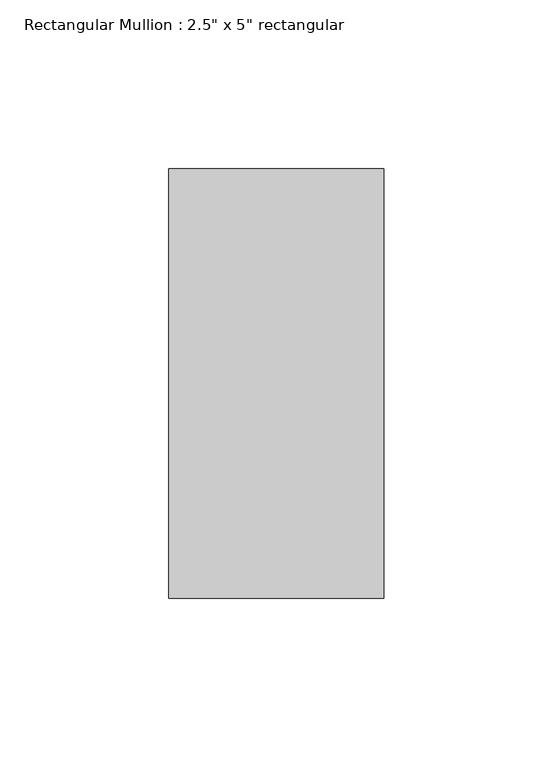
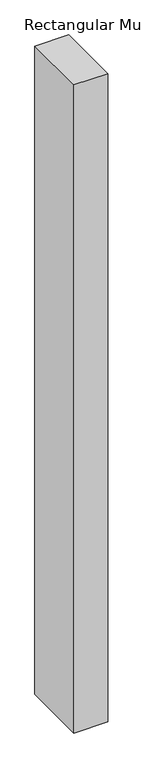
"""IFC4 building model written with IfcOpenShell, lengths in millimetres: member geometry."""

from ifc_helpers import new_model, si_unit, frame, origin, place, context, project, spatial, polyline, outline, extrude, source, transform, mapped, element, save


def member_d3e05364(model_context):
    return source(origin(), model_context, "Body", "SweptSolid", [
        extrude(outline(polyline([(0.0, 63.5), (0.0, -63.5), (-63.5, -63.5), (-63.5, 63.5), (0.0, 63.5)])), frame((0.0, 0.0, -1287.9932093), z_axis=(0.0, 0.0, 1.0), x_axis=(1.0, 0.0, 0.0)), (0.0, 0.0, 1.0), 1287.9932093),
    ])


if __name__ == "__main__":
    model = new_model("IFC4")
    model_context = context("Model", 3, world=origin())
    ifc_project = project(units=[si_unit("LENGTHUNIT", "METRE", prefix="MILLI")], contexts=[model_context])
    site = spatial("IfcSite", under=ifc_project)
    building = spatial("IfcBuilding", under=site)
    placement = place(None, origin())
    member_shape = member_d3e05364(model_context)
    element("IfcMember", 1, ObjectType="Rectangular Mullion : 2.5\" x 5\" rectangular", at=placement, inside=building, context=model_context, shape_type="MappedRepresentation", body=[
        mapped(member_shape, transform((0.0, 0.0, 0.0), x_axis=(1.0, 0.0, 0.0), y_axis=(0.0, 1.0, 0.0), z_axis=(0.0, 0.0, 1.0))),
    ])
    save(model, "model.ifc")

# Revit data of these elements
# Type "Rectangular Mullion : 2.5\" x 5\" rectangular"
#   built-in parameter 1007304 = 0.416667 (stored number, unit not read)
#   built-in parameter 1007301 = 0.104167 (stored number, unit not read)
#   built-in parameter 1007300 = 0.104167 (stored number, unit not read)
# Element 1 (IfcMember, "Rectangular Mullion : 2.5\" x 5\" rectangular")
#   Materials on its faces: "Aluminum"
# Materials
#   "Aluminum": class "Metal", colour RGB 247 247 247, transparency 0, Description = "Aluminum 6061", Cost = 0
